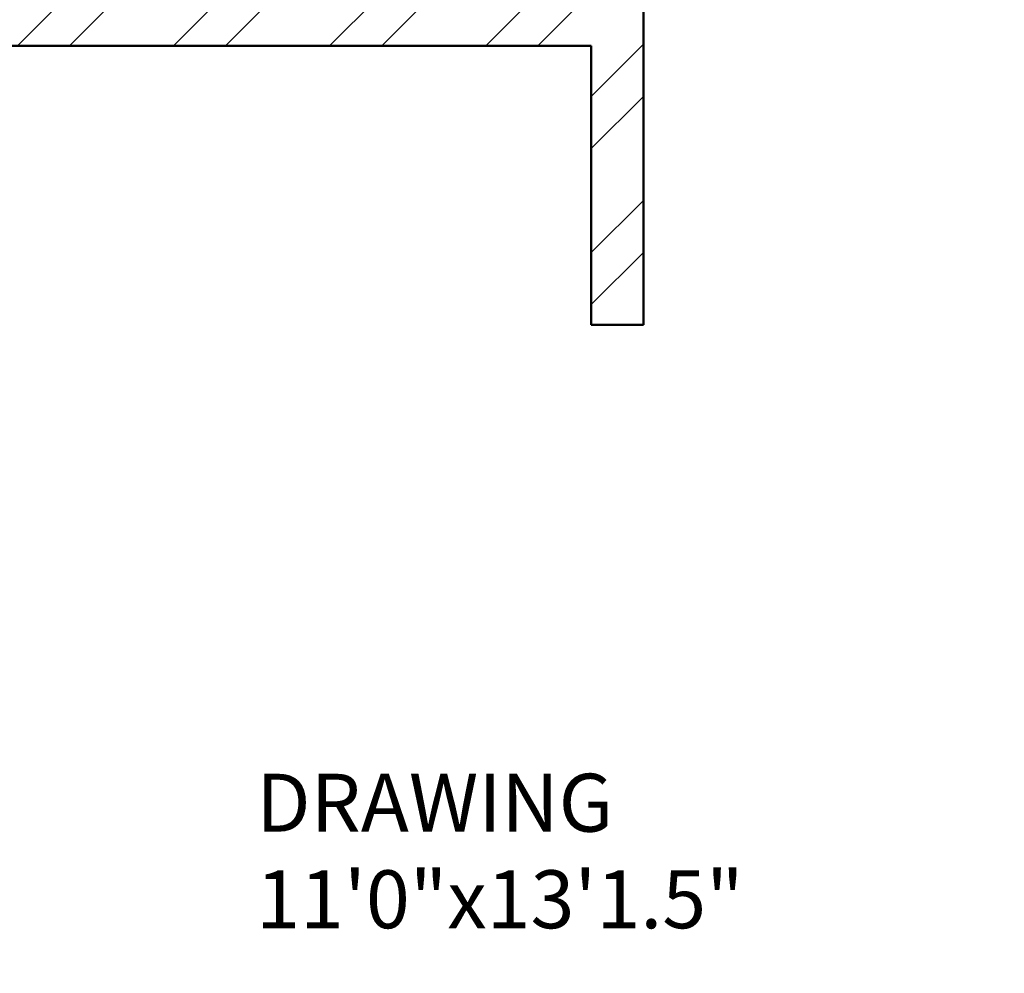
# Model space of a CAD drawing. Units: inches. Extents: x 963 to 2075, y 289 to 2657.
# Tile 87 of 98: x 1596 to 1681, y 2243 to 2325. Entities that reach past the tile are written whole.
import ezdxf

# ---------------------------------------------------------------- set-up
doc = ezdxf.new("R2010")
doc.units = ezdxf.units.IN
for name, color, linetype, lineweight in [('A-AREA-IDEN', 7, 'Continuous', 18), ('A-WALL', 7, 'Continuous', 50), ('A-WALL-PATT', 8, 'Continuous', 13)]:
    doc.layers.add(name, color=color, linetype=linetype, lineweight=lineweight)
doc.styles.get("Standard").update_dxf_attribs({"font": 'arial.ttf'})

msp = doc.modelspace()

# ---------------------------------------------------------------- hatches: boundary and pattern name
at = {"layer": 'A-WALL-PATT'}
h = msp.add_hatch(dxfattribs=at)
h.set_pattern_fill('ANSI32', color=256)
h.paths.add_polyline_path([(1296.922, 2558.318), (1203.922, 2558.318), (1203.922, 2493.818), (1191.533, 2493.818), (1191.533, 2489.318), (1211.063, 2489.318), (1211.063, 2492.02), (1211.063, 2493.818), (1208.422, 2493.818), (1208.422, 2553.818), (1292.422, 2553.818), (1292.422, 2538.863), (1296.922, 2538.863)])
h.paths.add_polyline_path([(1442.422, 2558.318), (1349.422, 2558.318), (1349.422, 2538.943), (1353.922, 2538.943), (1353.922, 2553.818), (1437.922, 2553.818), (1437.922, 2493.818), (1434.542, 2493.818), (1434.542, 2489.318), (1448.311, 2489.318), (1448.311, 2491.568), (1448.311, 2493.818), (1442.422, 2493.818)])
h.paths.add_polyline_path([(1415.554, 2491.568), (1415.554, 2493.818), (1340.941, 2493.818), (1340.941, 2489.318), (1371.922, 2489.318), (1371.922, 2378.318), (1367.596, 2378.318), (1367.596, 2373.818), (1371.922, 2373.818), (1371.922, 2355.185), (1376.422, 2355.185), (1376.422, 2489.318), (1415.554, 2489.318)])
h.paths.add_polyline_path([(1304.941, 2491.568), (1304.941, 2493.818), (1296.922, 2493.818), (1296.922, 2514.863), (1292.422, 2514.863), (1292.422, 2493.818), (1232.808, 2493.818), (1232.808, 2489.318), (1256.422, 2489.318), (1256.422, 2327.318), (1253.714, 2327.318), (1253.714, 2322.818), (1328.422, 2322.818), (1328.422, 2331.147), (1323.922, 2331.147), (1323.922, 2327.318), (1260.922, 2327.318), (1260.922, 2373.818), (1323.922, 2373.818), (1323.922, 2357.812), (1328.422, 2357.812), (1328.422, 2373.818), (1346.007, 2373.818), (1346.007, 2376.068), (1346.007, 2378.318), (1260.922, 2378.318), (1260.922, 2489.318), (1304.941, 2489.318)])
h.paths.add_polyline_path([(1226.654, 2327.318), (1124.422, 2327.318), (1124.422, 2347.447), (1119.922, 2347.447), (1119.922, 2322.818), (1163.422, 2322.818), (1163.422, 2305.435), (1165.672, 2305.435), (1167.922, 2305.435), (1167.922, 2322.818), (1226.654, 2322.818), (1226.654, 2325.068)])
h.paths.add_polyline_path([(1095.922, 2489.318), (1124.422, 2489.318), (1131.533, 2489.318), (1131.533, 2491.568), (1131.533, 2493.818), (1119.922, 2493.818), (1091.422, 2493.818), (1091.422, 2417.318), (1095.922, 2417.318), (1119.922, 2417.318), (1119.922, 2407.447), (1124.422, 2407.447), (1124.422, 2421.818), (1095.922, 2421.818)])
h.paths.add_polyline_path([(1512.922, 2558.318), (1508.422, 2558.318), (1508.422, 2493.818), (1503.401, 2493.818), (1503.401, 2489.318), (1508.422, 2489.318), (1508.422, 2327.318), (1376.422, 2327.318), (1376.422, 2330.273), (1371.922, 2330.273), (1371.922, 2298.744), (1376.422, 2298.744), (1376.422, 2322.818), (1508.422, 2322.818), (1508.422, 2165.318), (1504.255, 2165.318), (1504.255, 2160.818), (1508.422, 2160.818), (1508.422, 2108.318), (1512.922, 2108.318), (1512.922, 2160.818), (1516.182, 2160.818), (1516.182, 2163.068), (1516.182, 2165.318), (1512.922, 2165.318), (1512.922, 2322.818), (1644.922, 2322.818), (1644.922, 2298.744), (1649.422, 2298.744), (1649.422, 2322.818), (1649.422, 2330.944), (1647.172, 2330.944), (1644.922, 2330.944), (1644.922, 2327.318), (1512.922, 2327.318), (1512.922, 2489.318), (1516.759, 2489.318), (1516.759, 2491.568), (1516.759, 2493.818), (1512.922, 2493.818)])
h.paths.add_polyline_path([(1671.922, 2558.318), (1578.922, 2558.318), (1578.922, 2493.818), (1573.526, 2493.818), (1573.526, 2489.318), (1586.537, 2489.318), (1586.537, 2491.568), (1586.537, 2493.818), (1583.422, 2493.818), (1583.422, 2553.818), (1667.422, 2553.818), (1667.422, 2541.109), (1671.922, 2541.109)])
h.paths.add_polyline_path([(1681.257, 2493.818), (1671.922, 2493.818), (1671.922, 2517.109), (1667.422, 2517.109), (1667.422, 2493.818), (1610.218, 2493.818), (1610.218, 2489.318), (1644.922, 2489.318), (1644.922, 2357.865), (1649.422, 2357.865), (1649.422, 2373.818), (1652.203, 2373.818), (1652.203, 2375.827), (1652.203, 2378.318), (1649.422, 2378.318), (1649.422, 2489.318), (1681.257, 2489.318), (1681.257, 2491.568)])
h.paths.add_polyline_path([(1821.922, 2558.318), (1728.922, 2558.318), (1728.922, 2541), (1733.422, 2541), (1733.422, 2553.818), (1817.422, 2553.818), (1817.422, 2493.818), (1813.507, 2493.818), (1813.507, 2489.318), (1830.078, 2489.318), (1830.078, 2491.568), (1830.078, 2493.818), (1821.922, 2493.818)])
h.paths.add_polyline_path([(1794.244, 2493.818), (1717.257, 2493.818), (1717.257, 2489.318), (1760.422, 2489.318), (1760.422, 2378.318), (1674.401, 2378.318), (1674.401, 2373.818), (1692.922, 2373.818), (1692.922, 2356.954), (1697.422, 2356.954), (1697.422, 2373.818), (1760.422, 2373.818), (1760.422, 2327.318), (1697.422, 2327.318), (1697.422, 2333.341), (1692.922, 2333.341), (1692.922, 2322.818), (1768.037, 2322.818), (1768.037, 2325.068), (1768.037, 2327.318), (1764.922, 2327.318), (1764.922, 2489.318), (1794.244, 2489.318)])
h.paths.add_polyline_path([(1733.422, 2517), (1728.922, 2517), (1728.922, 2493.818), (1733.422, 2493.818)], flags=17)
h.paths.add_polyline_path([(1929.922, 2493.818), (1890.078, 2493.818), (1890.078, 2489.318), (1896.922, 2489.318), (1925.422, 2489.318), (1925.422, 2421.818), (1896.922, 2421.818), (1896.922, 2408.318), (1901.422, 2408.318), (1901.422, 2417.318), (1925.422, 2417.318), (1929.922, 2417.318)])
h.paths.add_polyline_path([(1901.422, 2348.318), (1896.922, 2348.318), (1896.922, 2327.318), (1800.423, 2327.318), (1800.423, 2322.818), (1853.422, 2322.818), (1853.422, 2309.453), (1857.922, 2309.453), (1857.922, 2322.818), (1901.422, 2322.818)])
h.paths.add_polyline_path([(1857.922, 2249.453), (1853.422, 2249.453), (1853.422, 2214.818), (1686.309, 2214.818), (1686.309, 2210.318), (1853.422, 2210.318), (1853.422, 2202.134), (1857.922, 2202.134), (1857.922, 2210.318)])
h.paths.add_polyline_path([(1857.922, 2142.134), (1853.422, 2142.134), (1853.422, 2115.422), (1841.422, 2115.422), (1841.422, 2088.531), (1841.422, 2046.949), (1845.922, 2046.949), (1845.922, 2110.922), (1905.922, 2110.922), (1905.922, 2092.517), (1910.422, 2092.517), (1910.422, 2115.422), (1857.922, 2115.422)])
h.paths.add_polyline_path([(1532.436, 1482.342), (1573.456, 1482.342), (1573.456, 1501), (1532.436, 1501)], flags=9)
h.paths.add_polyline_path([(1438.658, 1486.302), (1479.678, 1486.302), (1479.678, 1504.96), (1438.658, 1504.96)], flags=9)
h.paths.add_polyline_path([(1411.215, 1365.308), (1659.139, 1365.308), (1659.139, 1402.401), (1411.215, 1402.401)], flags=9)
h.paths.add_polyline_path([(1185.671, 2296.298), (1248.16, 2296.298), (1248.16, 2314.955), (1185.671, 2314.955)], flags=9)
h.paths.add_polyline_path([(1177.31, 2187.35), (1216.15, 2187.35), (1216.15, 2206.007), (1177.31, 2206.007)], flags=9)
h.paths.add_polyline_path([(1295.101, 1602.083), (1328.26, 1602.083), (1328.26, 1620.741), (1295.101, 1620.741)], flags=9)
h.paths.add_polyline_path([(1525.126, 2005.99), (1558.39, 2005.99), (1558.39, 2024.648), (1525.126, 2024.648)], flags=9)
h.paths.add_polyline_path([(1459.606, 1977.125), (1472.195, 1977.125), (1472.195, 1987.429), (1459.606, 1987.429)], flags=9)
h.paths.add_polyline_path([(1467.815, 2053.676), (1480.018, 2053.676), (1480.018, 2063.979), (1467.815, 2063.979)], flags=9)
h.paths.add_polyline_path([(1555.184, 2119.02), (1584.563, 2119.02), (1584.563, 2137.678), (1555.184, 2137.678)], flags=25)
h.paths.add_polyline_path([(1405.389, 2115.291), (1444.478, 2115.291), (1444.478, 2133.948), (1405.389, 2133.948)], flags=25)
h.paths.add_polyline_path([(1698.482, 2004.259), (1727.695, 2004.259), (1727.695, 2022.916), (1698.482, 2022.916)], flags=9)
h.paths.add_polyline_path([(1612.158, 1972.855), (1629.016, 1972.855), (1629.016, 1983.159), (1612.158, 1983.159)], flags=9)
h.paths.add_polyline_path([(1608.289, 2060.036), (1625.147, 2060.036), (1625.147, 2070.34), (1608.289, 2070.34)], flags=9)
h.paths.add_polyline_path([(1527.954, 1684.402), (1566.795, 1684.402), (1566.795, 1703.06), (1527.954, 1703.06)], flags=9)
h.paths.add_polyline_path([(1422.792, 1683.59), (1461.633, 1683.59), (1461.633, 1702.247), (1422.792, 1702.247)], flags=9)
h.paths.add_polyline_path([(1531.262, 1732.459), (1574.015, 1732.459), (1574.015, 1751.116), (1531.262, 1751.116)], flags=9)
h.paths.add_polyline_path([(1402.872, 1732.845), (1439.799, 1732.845), (1439.799, 1751.502), (1402.872, 1751.502)], flags=9)
h.paths.add_polyline_path([(1243.122, 1923.132), (1281.962, 1923.132), (1281.962, 1941.79), (1243.122, 1941.79)], flags=9)
h.paths.add_polyline_path([(1181.752, 1792.268), (1244.241, 1792.268), (1244.241, 1810.926), (1181.752, 1810.926)], flags=9)
h.paths.add_polyline_path([(1265.822, 1670.3), (1316.071, 1670.3), (1316.071, 1688.957), (1265.822, 1688.957)], flags=9)
h.paths.add_polyline_path([(1140.263, 1676.054), (1179.104, 1676.054), (1179.104, 1694.711), (1140.263, 1694.711)], flags=9)
h.paths.add_polyline_path([(1107.49, 1490.889), (1143.374, 1490.889), (1143.374, 1509.546), (1107.49, 1509.546)], flags=9)
h.paths.add_polyline_path([(1217.584, 1483.899), (1246.741, 1483.899), (1246.741, 1502.556), (1217.584, 1502.556)], flags=9)
h.paths.add_polyline_path([(1389.21, 1486.919), (1418.367, 1486.919), (1418.367, 1505.576), (1389.21, 1505.576)], flags=9)
h.paths.add_polyline_path([(1672.208, 1602.083), (1705.366, 1602.083), (1705.366, 1620.741), (1672.208, 1620.741)], flags=9)
h.paths.add_polyline_path([(1752.082, 1522.638), (1781.24, 1522.638), (1781.24, 1541.295), (1752.082, 1541.295)], flags=9)
h.paths.add_polyline_path([(1848.275, 1491.26), (1884.158, 1491.26), (1884.158, 1509.918), (1848.275, 1509.918)], flags=9)
h.paths.add_polyline_path([(1822.47, 1685.62), (1861.31, 1685.62), (1861.31, 1704.278), (1822.47, 1704.278)], flags=9)
h.paths.add_polyline_path([(1713.195, 1672.232), (1763.444, 1672.232), (1763.444, 1690.889), (1713.195, 1690.889)], flags=9)
h.paths.add_polyline_path([(1736.619, 1790.578), (1799.109, 1790.578), (1799.109, 1809.235), (1736.619, 1809.235)], flags=9)
h.paths.add_polyline_path([(1691.491, 1916.355), (1730.332, 1916.355), (1730.332, 1935.013), (1691.491, 1935.013)], flags=9)
h.paths.add_polyline_path([(1764.872, 1973.922), (1794.306, 1973.922), (1794.306, 1992.58), (1764.872, 1992.58)], flags=9)
h.paths.add_polyline_path([(1767.854, 2034.017), (1797.288, 2034.017), (1797.288, 2052.674), (1767.854, 2052.674)], flags=9)
h.paths.add_polyline_path([(1851.593, 2060.331), (1880.751, 2060.331), (1880.751, 2078.989), (1851.593, 2078.989)], flags=25)
h.paths.add_polyline_path([(1688.491, 2086.874), (1727.332, 2086.874), (1727.332, 2105.531), (1688.491, 2105.531)], flags=9)
h.paths.add_polyline_path([(1537.743, 2293.581), (1580.495, 2293.581), (1580.495, 2312.239), (1537.743, 2312.239)], flags=25)
h.paths.add_polyline_path([(1425.587, 2296.109), (1468.34, 2296.109), (1468.34, 2314.766), (1425.587, 2314.766)], flags=25)
h.paths.add_polyline_path([(1278.518, 2004.184), (1307.72, 2004.184), (1307.72, 2022.841), (1278.518, 2022.841)], flags=9)
h.paths.add_polyline_path([(1193.282, 1973.635), (1222.715, 1973.635), (1222.715, 1992.292), (1193.282, 1992.292)], flags=9)
h.paths.add_polyline_path([(1192.411, 2040.577), (1221.845, 2040.577), (1221.845, 2059.234), (1192.411, 2059.234)], flags=9)
h.paths.add_polyline_path([(1130.603, 1951.393), (1159.76, 1951.393), (1159.76, 1970.05), (1130.603, 1970.05)], flags=9)
h.paths.add_polyline_path([(1132.827, 2052.494), (1161.984, 2052.494), (1161.984, 2071.151), (1132.827, 2071.151)], flags=9)
h.paths.add_polyline_path([(1265.128, 2334.619), (1315.377, 2334.619), (1315.377, 2353.277), (1265.128, 2353.277)], flags=25)
h.paths.add_polyline_path([(1136.741, 2330.785), (1175.582, 2330.785), (1175.582, 2349.443), (1136.741, 2349.443)], flags=9)
h.paths.add_polyline_path([(1287.422, 2417.204), (1320.58, 2417.204), (1320.58, 2435.861), (1287.422, 2435.861)], flags=25)
h.paths.add_polyline_path([(1430.988, 2329.159), (1469.828, 2329.159), (1469.828, 2347.816), (1430.988, 2347.816)], flags=25)
h.paths.add_polyline_path([(1525.424, 2329.213), (1564.264, 2329.213), (1564.264, 2347.87), (1525.424, 2347.87)], flags=25)
h.paths.add_polyline_path([(1684.525, 2382.799), (1717.683, 2382.799), (1717.683, 2401.457), (1684.525, 2401.457)], flags=25)
h.paths.add_polyline_path([(1704.805, 2340.293), (1755.054, 2340.293), (1755.054, 2358.95), (1704.805, 2358.95)], flags=25)
h.paths.add_polyline_path([(1694.113, 2287.757), (1756.602, 2287.757), (1756.602, 2306.414), (1694.113, 2306.414)], flags=9)
h.paths.add_polyline_path([(1815.778, 2329.861), (1854.618, 2329.861), (1854.618, 2348.518), (1815.778, 2348.518)], flags=9)
h.paths.add_polyline_path([(1842.873, 2514.256), (1878.756, 2514.256), (1878.756, 2532.914), (1842.873, 2532.914)], flags=9)
h.paths.add_polyline_path([(1769.513, 2531.447), (1798.671, 2531.447), (1798.671, 2550.104), (1769.513, 2550.104)], flags=25)
h.paths.add_polyline_path([(1594.772, 2518.468), (1623.93, 2518.468), (1623.93, 2537.125), (1594.772, 2537.125)], flags=25)
h.paths.add_polyline_path([(1520.723, 2516.185), (1556.606, 2516.185), (1556.606, 2534.842), (1520.723, 2534.842)], flags=25)
h.paths.add_polyline_path([(1464.456, 2516.694), (1500.34, 2516.694), (1500.34, 2535.351), (1464.456, 2535.351)], flags=25)
h.paths.add_polyline_path([(1365.696, 2528.97), (1394.854, 2528.97), (1394.854, 2547.627), (1365.696, 2547.627)], flags=25)
h.paths.add_polyline_path([(1222.838, 2516.231), (1251.995, 2516.231), (1251.995, 2534.889), (1222.838, 2534.889)], flags=25)
h.paths.add_polyline_path([(1104.545, 2509.6), (1140.429, 2509.6), (1140.429, 2528.257), (1104.545, 2528.257)], flags=9)

# ---------------------------------------------------------------- linework, layer by layer
at = {"layer": 'A-WALL'}
for p, q in [((1649.422, 2330.944), (1649.422, 2322.818)), ((1512.922, 2322.818), (1644.922, 2322.818)), ((1644.922, 2322.818), (1644.922, 2298.744)), ((1649.422, 2322.818), (1649.422, 2298.744)), ((1644.922, 2298.744), (1649.422, 2298.744))]:
    msp.add_line(p, q, dxfattribs=at)

# ---------------------------------------------------------------- texts
at = {"layer": 'A-AREA-IDEN', "insert": (1616.021, 2259.989), "char_height": 5, "attachment_point": 1}
msp.add_mtext_dynamic_manual_height_columns('DRAWING\\P11\'0"x13\'1.5"', width=153.56751, gutter_width=12.5, heights=[0], dxfattribs=at)

doc.saveas('drawing.dxf')
